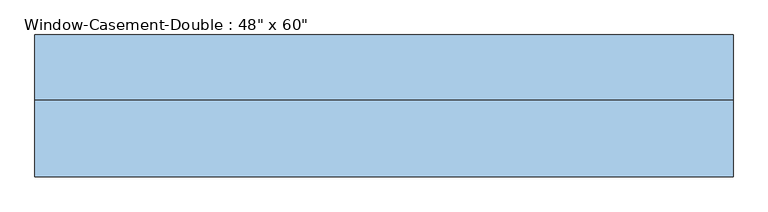
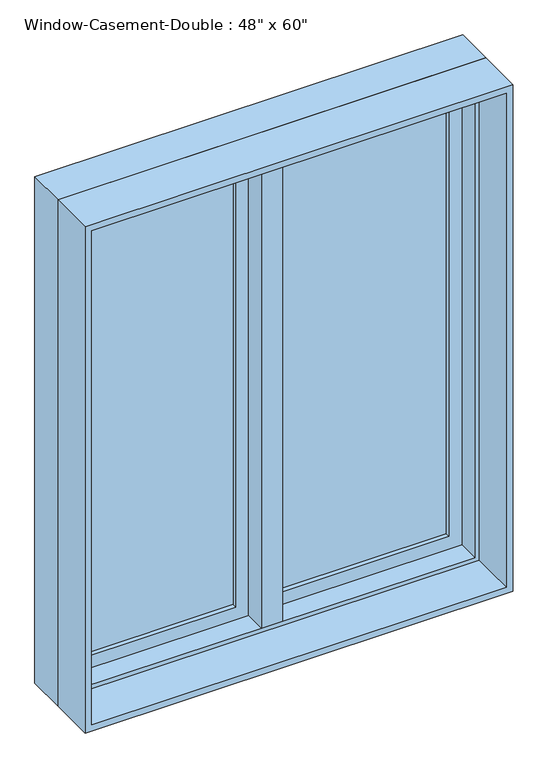
"""IFC4 building model written with IfcOpenShell, lengths in millimetres: window geometry."""

from ifc_helpers import new_model, si_unit, frame, origin, place, context, project, spatial, polyline, outline, extrude, faceted_brep, source, transform, mapped, element, save


def window_8377141f(model_context):
    return source(origin(), model_context, "Body", "SolidModel", [
        faceted_brep([(9.525, 133.35, 2425.7), (-9.525, 133.35, 2425.7), (-9.525, 82.55, 2425.7), (9.525, 82.55, 2425.7), (9.525, 133.35, 927.1), (9.525, 82.55, 927.1), (-9.525, 82.55, 927.1), (-9.525, 133.35, 927.1), (-9.525, 82.55, 946.15), (-9.525, 82.55, 2406.65), (-30.1625, 82.55, 946.15), (-30.1625, 82.55, 2406.65), (-30.1625, 19.05, 946.15), (-30.1625, 19.05, 2406.65), (30.1625, 19.05, 946.15), (30.1625, 19.05, 2406.65), (30.1625, 82.55, 946.15), (30.1625, 82.55, 2406.65), (9.525, 82.55, 946.15), (9.525, 82.55, 2406.65)], [[[0, 1, 2, 3]], [[4, 5, 6, 7]], [[1, 0, 4, 7]], [[2, 1, 7, 6, 8, 9]], [[9, 8, 10, 11]], [[11, 10, 12, 13]], [[13, 12, 14, 15]], [[15, 14, 16, 17]], [[17, 16, 18, 19]], [[0, 3, 19, 18, 5, 4]], [[18, 8, 6, 5]], [[9, 19, 3, 2]], [[8, 18, 16, 14, 12, 10]], [[19, 9, 11, 13, 15, 17]]]),
        extrude(outline(polyline([(-66.675, 114.3), (-66.675, 107.95), (-539.75, 107.95), (-539.75, 114.3), (-66.675, 114.3)])), frame((0.0, 0.0, 984.25), z_axis=(0.0, 0.0, 1.0), x_axis=(1.0, 0.0, 0.0)), (0.0, 0.0, 1.0), 1384.3),
        extrude(outline(polyline([(-539.75, 95.25), (-539.75, 101.6), (-66.675, 101.6), (-66.675, 95.25), (-539.75, 95.25)])), frame((0.0, 0.0, 984.25), z_axis=(0.0, 0.0, 1.0), x_axis=(1.0, 0.0, 0.0)), (0.0, 0.0, 1.0), 1384.3),
        extrude(outline(polyline([(539.75, 114.3), (539.75, 107.95), (66.675, 107.95), (66.675, 114.3), (539.75, 114.3)])), frame((0.0, 0.0, 984.25), z_axis=(0.0, 0.0, 1.0), x_axis=(1.0, 0.0, 0.0)), (0.0, 0.0, 1.0), 1384.3),
        extrude(outline(polyline([(66.675, 95.25), (66.675, 101.6), (539.75, 101.6), (539.75, 95.25), (66.675, 95.25)])), frame((0.0, 0.0, 984.25), z_axis=(0.0, 0.0, 1.0), x_axis=(1.0, 0.0, 0.0)), (0.0, 0.0, 1.0), 1384.3),
        extrude(outline(polyline([(2425.7, -596.9), (927.1, -596.9), (927.1, -9.525), (2425.7, -9.525), (2425.7, -596.9)]), holes=[polyline([(2368.55, -66.675), (984.25, -66.675), (984.25, -539.75), (2368.55, -539.75), (2368.55, -66.675)])]), frame((0.0, 82.55, 0.0), z_axis=(0.0, 1.0, 0.0), x_axis=(0.0, 0.0, 1.0)), (0.0, 0.0, 1.0), 44.45),
        extrude(outline(polyline([(927.1, 596.9), (2425.7, 596.9), (2425.7, 9.525), (927.1, 9.525), (927.1, 596.9)]), holes=[polyline([(984.25, 66.675), (2368.55, 66.675), (2368.55, 539.75), (984.25, 539.75), (984.25, 66.675)])]), frame((0.0, 82.55, 0.0), z_axis=(0.0, 1.0, 0.0), x_axis=(0.0, 0.0, 1.0)), (0.0, 0.0, 1.0), 44.45),
        extrude(outline(polyline([(2438.4, -609.6), (914.4, -609.6), (914.4, 609.6), (2438.4, 609.6), (2438.4, -609.6)]), holes=[polyline([(2419.35, 590.55), (933.45, 590.55), (933.45, -590.55), (2419.35, -590.55), (2419.35, 590.55)])]), frame((0.0, -114.3, 0.0), z_axis=(0.0, 1.0, 0.0), x_axis=(0.0, 0.0, 1.0)), (0.0, 0.0, 1.0), 133.35),
        faceted_brep([(577.85, 82.55, 2406.65), (577.85, 19.05, 2406.65), (-577.85, 19.05, 2406.65), (-577.85, 82.55, 2406.65), (596.9, 133.35, 2425.7), (596.9, 82.55, 2425.7), (-596.9, 82.55, 2425.7), (-596.9, 133.35, 2425.7), (609.6, 19.05, 2438.4), (609.6, 133.35, 2438.4), (-609.6, 133.35, 2438.4), (-609.6, 19.05, 2438.4), (-577.85, 19.05, 946.15), (-577.85, 82.55, 946.15), (-596.9, 82.55, 927.1), (-596.9, 133.35, 927.1), (-609.6, 133.35, 914.4), (-609.6, 19.05, 914.4), (577.85, 19.05, 946.15), (577.85, 82.55, 946.15), (596.9, 82.55, 927.1), (596.9, 133.35, 927.1), (609.6, 133.35, 914.4), (609.6, 19.05, 914.4)], [[[0, 1, 2, 3]], [[4, 5, 6, 7]], [[8, 9, 10, 11]], [[3, 2, 12, 13]], [[7, 6, 14, 15]], [[11, 10, 16, 17]], [[13, 12, 18, 19]], [[15, 14, 20, 21]], [[17, 16, 22, 23]], [[11, 17, 23, 8], [1, 18, 12, 2]], [[19, 18, 1, 0]], [[5, 20, 14, 6], [3, 13, 19, 0]], [[21, 20, 5, 4]], [[23, 22, 9, 8]], [[9, 22, 16, 10], [7, 15, 21, 4]]]),
    ])


if __name__ == "__main__":
    model = new_model("IFC4")
    model_context = context("Model", 3, world=origin())
    ifc_project = project(units=[si_unit("LENGTHUNIT", "METRE", prefix="MILLI")], contexts=[model_context])
    site = spatial("IfcSite", under=ifc_project)
    building = spatial("IfcBuilding", under=site)
    placement = place(None, origin())
    window_shape = window_8377141f(model_context)
    element("IfcWindow", 1, ObjectType="Window-Casement-Double : 48\" x 60\"", at=placement, inside=building, context=model_context, shape_type="MappedRepresentation", body=[
        mapped(window_shape, transform((0.0, 0.0, 0.0), x_axis=(1.0, 0.0, 0.0), y_axis=(0.0, 1.0, 0.0), z_axis=(0.0, 0.0, 1.0))),
    ])
    save(model, "model.ifc")

# Revit data of these elements
# Type "Window-Casement-Double : 48\" x 60\""
#   Type Mark = "16"
#   Fire Rating = "0.5h"
#   Assembly Code = "B2020100"
#   Analytic Construction = "Double glazing - domestic"
#   Frame Extension [instance default] = 0' - 0 1/4"
#   Window Inset [instance default] = 0' - 0"
#   Wall Thickness [instance default] = 0' - 6"
#   Interior Wall Closure [instance default] = 0' - 2 1/4"
#   Half Width = 2' - 0"
#   Visual Light Transmittance = 0.81
#   Thermal Resistance (R) = 1.8146 (h·ft²·°F)/BTU
#   Solar Heat Gain Coefficient = 0.76
#   Rough Width = 4' - 0 1/2"
#   Rough Height = 5' - 0 1/2"
#   Height = 5' - 0"
#   Heat Transfer Coefficient (U) = 0.5511 BTU/(h·ft²·°F)
#   Exterior Wall Closure [instance default] = 0' - 1 1/4"
#   Extension Jamb [instance default] = 0' - 2 1/4"
#   Default Sill Height = 3' - 0"
#   Width = 4' - 0"
#   Define Thermal Properties by = 0
#   Muntin Visibility = yes
#   Interior Trim Visibility [instance default] = yes
#   Exterior Trim Visibility [instance default] = yes
#   Extension Jamb Visibility [instance default] = yes
#   Interior Trim Material = Wood - Stained
#   Muntin Pattern = Muntin Pattern_2x2 : Muntin Pattern_2x2
#   Interior Trim = Trim-Window-Interior-Flat : Picture Frame
#   Interior Frame Material = Wood - Stained
#   Glass Panel Material = Glass
#   Exterior Trim Material = Clad - White
#   Exterior Trim = Trim-Window-Exterior-Flat : with Sill
#   Exterior Frame Material = Clad - White
#   Wall Closure = (empty or 0)
# Element 1 (IfcWindow, "Window-Casement-Double : 48\" x 60\"")
#   Wall Thickness = 0' - 9"
#   Extension Jamb = 0' - 5 1/4"
#   Materials on its faces: "Wood - Stained", "Glass", "Clad - White"
# Materials
#   "Wood - Stained": class "Wood", colour RGB 224 178 126, transparency 0, Cost = 0
#   "Glass": class "Glass", colour RGB 0 128 192, transparency 0.75, Description = "Soda Lime Glass", Cost = 0
#   "Clad - White": class "Wood", colour RGB 242 242 238, transparency 0, Cost = 0
